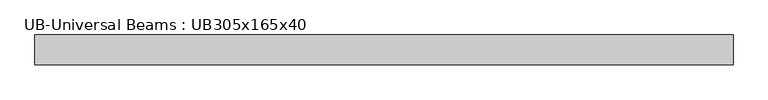
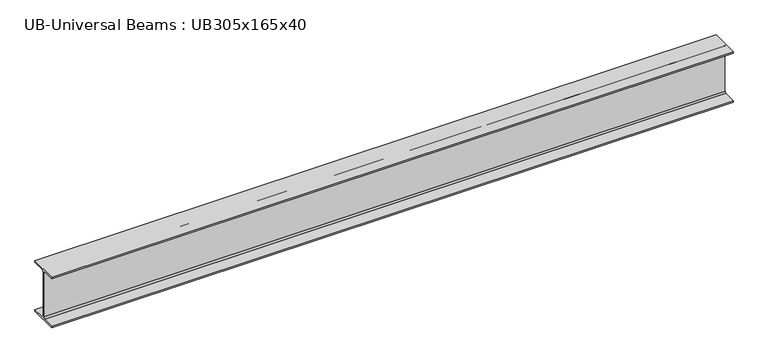
"""IFC4 building model written with IfcOpenShell, lengths in millimetres: beam geometry, UB-Universal Beams : UB305x165x40."""

from ifc_helpers import new_model, si_unit, point, frame, frame_2d, origin, place, context, project, spatial, polyline, circle_curve, trimmed, segment, composite_curve, outline, extrude, source, transform, mapped, element, save


def ub_universal_beams_ub305x165x40_c956ba20(model_context):
    return source(origin(), model_context, "Body", "SweptSolid", [
        extrude(outline(composite_curve([segment(polyline([(82.5, -141.5), (82.5, -151.7), (-82.5, -151.7), (-82.5, -141.5), (-11.9, -141.5)]), True, "CONTINUOUS"), segment(trimmed(circle_curve(frame_2d((-11.9, -132.6)), 8.9), [point((-11.9, -141.5))], [point((-3.0, -132.6))], True, "CARTESIAN"), True, "CONTINUOUS"), segment(polyline([(-3.0, -132.6), (-3.0, 132.6)]), True, "CONTINUOUS"), segment(trimmed(circle_curve(frame_2d((-11.9, 132.6)), 8.9), [point((-3.0, 132.6))], [point((-11.9, 141.5))], True, "CARTESIAN"), True, "CONTINUOUS"), segment(polyline([(-11.9, 141.5), (-82.5, 141.5), (-82.5, 151.7), (82.5, 151.7), (82.5, 141.5), (11.9, 141.5)]), True, "CONTINUOUS"), segment(trimmed(circle_curve(frame_2d((11.9, 132.6)), 8.9), [point((11.9, 141.5))], [point((3.0, 132.6))], True, "CARTESIAN"), True, "CONTINUOUS"), segment(polyline([(3.0, 132.6), (3.0, -132.6)]), True, "CONTINUOUS"), segment(trimmed(circle_curve(frame_2d((11.9, -132.6)), 8.9), [point((3.0, -132.6))], [point((11.9, -141.5))], True, "CARTESIAN"), True, "CONTINUOUS"), segment(polyline([(11.9, -141.5), (82.5, -141.5)]), True, "CONTINUOUS")], self_intersect=False)), frame((-2120.25, 0.0, 0.0), z_axis=(1.0, 0.0, 0.0), x_axis=(0.0, 1.0, 0.0)), (0.0, 0.0, 1.0), 3860.0),
    ])


if __name__ == "__main__":
    model = new_model("IFC4")
    model_context = context("Model", 3, world=origin())
    ifc_project = project(units=[si_unit("LENGTHUNIT", "METRE", prefix="MILLI")], contexts=[model_context])
    site = spatial("IfcSite", under=ifc_project)
    building = spatial("IfcBuilding", under=site)
    placement = place(None, origin())
    ub_universal_beams_ub305x165x40_shape = ub_universal_beams_ub305x165x40_c956ba20(model_context)
    element("IfcBeam", 1, ObjectType="UB-Universal Beams : UB305x165x40", at=placement, inside=building, context=model_context, shape_type="MappedRepresentation", body=[
        mapped(ub_universal_beams_ub305x165x40_shape, transform((0.0, 0.0, 0.0), x_axis=(1.0, 0.0, 0.0), y_axis=(0.0, 1.0, 0.0), z_axis=(0.0, 0.0, 1.0))),
    ])
    save(model, "model.ifc")

# Revit data of these elements
# Type "UB-Universal Beams : UB305x165x40"
#   Section Name Key = "UB305X165X40"
#   Width = 16.5 cm
#   Web Thickness = 0.6 cm
#   Web Fillet = 0.89 cm
#   Warping Constant = 164000.0 cm⁶
#   Torsional Moment of Inertia = 14.70 cm⁴
#   Section Area = 51.3 cm²
#   Plastic Modulus weak axis = 142.0 cm³
#   Plastic Modulus strong axis = 623.0 cm³
#   Nominal Weight = 40.2999 kgf/m
#   Moment of Inertia weak axis = 764.00 cm⁴
#   Moment of Inertia strong axis = 8503.00 cm⁴
#   Height = 30.34 cm
#   Flange Thickness = 1.02 cm
#   Elastic Modulus weak axis = 92.6 cm³
#   Elastic Modulus strong axis = 560.0 cm³
#   Centroid Vertical = 15.17 cm
#   Centroid Horizontal = 8.25 cm
#   Bolt Spacing = 9.0 cm
#   Length [instance default] = 1500 mm
#   Structural Material [instance default] = Metal - Steel 43-275
#   Type Comments = ""
#   Assembly Code = ""
# Element 1 (IfcBeam, "UB-Universal Beams : UB305x165x40")
#   Materials on its faces: "Metal - Steel 43-275"
# Materials
#   "Metal - Steel 43-275": class "Metal", colour RGB 247 247 247, transparency 0, Cost = 0
